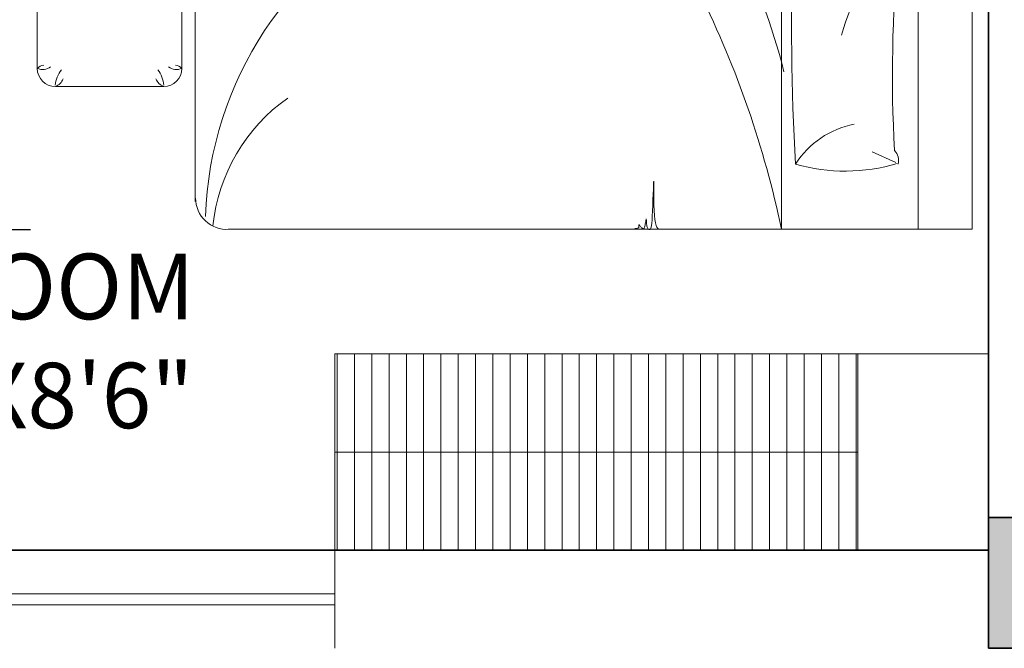
# Model space of a CAD drawing. Units: inches. Extents: x 3321 to 5237, y 11 to 1752.
# Tile 16 of 43: x 4367 to 4458, y 1172 to 1230. Entities that reach past the tile are written whole.
import ezdxf

# ---------------------------------------------------------------- set-up
doc = ezdxf.new("R2010")
doc.units = ezdxf.units.IN
for name, color, linetype, lineweight in [('A-ANNO-DIMS', 2, 'Continuous', 18), ('A-AREA-IDEN', 7, 'Continuous', 18), ('A-COLS', 1, 'Continuous', 35), ('A-FLOR-CASE', 8, 'Continuous', 18), ('A-FLOR-CASE-PATT', 8, 'Continuous', 13), ('A-GLAZ', 5, 'Continuous', 18), ('A-WALL', 7, 'Continuous', 35), ('FUR', 42, 'Continuous', 18)]:
    doc.layers.add(name, color=color, linetype=linetype, lineweight=lineweight)
doc.styles.get("Standard").update_dxf_attribs({"font": 'arial.ttf'})
doc.dimstyles.new('ISO-25', dxfattribs={"dimtxt": 9, "dimasz": 2.5, "dimexe": 1.25, "dimexo": 0.625, "dimtad": 1, "dimdec": 1, "dimlunit": 3, "dimtxsty": 'Standard', "dimcen": 2.5, "dimclrd": 4, "dimclre": 4, "dimclrt": 256, "dimadec": 0, "dimazin": 0, "dimtfac": 1, "dimtdec": 1, "dimtmove": 0, "dimatfit": 3, "dimfxl": 1, "dimarcsym": 0})

# ---------------------------------------------------------------- blocks, each defined once
blk = doc.blocks.new('*X127')
at = {"color": 0}
for p, q in [((3155.9, 8182.9), (3155.9, 8182.9)), ((3147.8, 8143.4), (3147.8, 8143.4)), ((3283, 8049.6), (3283, 8049.6)), ((3209.5, 8023.9), (3209.5, 8023.9)), ((3251.6, 7997), (3251.6, 7997)), ((3154.1, 7950.7), (3154.1, 7950.7))]:
    blk.add_line(p, q, dxfattribs=at)
blk = doc.blocks.new('*X126')
at = {"color": 0}
for p, q in [((3155.9, 8182.9), (3155.9, 8182.9)), ((3139.8, 7939.7), (3139.8, 7939.7))]:
    blk.add_line(p, q, dxfattribs=at)
blk = doc.blocks.new('*X125')
at = {"color": 0}
for p, q in [((3155.9, 8182.9), (3155.9, 8182.9)), ((3139.8, 7939.7), (3139.8, 7939.7))]:
    blk.add_line(p, q, dxfattribs=at)
blk = doc.blocks.new('*X124')
at = {"color": 0}
for p, q in [((3163, 7776.2), (3163, 7776.2)), ((3422.2, 7761.3), (3422.2, 7761.3)), ((3244.3, 7698.6), (3244.3, 7698.6)), ((3340.3, 7689.4), (3340.3, 7689.4)), ((3236.2, 7675.7), (3236.2, 7675.7))]:
    blk.add_line(p, q, dxfattribs=at)
blk = doc.blocks.new('BED1')
for p, q in [((0, -1000), (0, 800)), ((150, 800), (0, 800)), ((150, 800), (150, -1000)), ((2058.7, 800), (150, 800)), ((528, 800), (528, -1000)), ((211.8, 614.9), (277.5, 585.4)), ((2537.2, 404.9), (2237.2, 404.9)), ((2187.2, 354.9), (2187.2, -545.1)), ((2587.2, -545.1), (2587.2, 354.9)), ((2566.3, 178.5), (2565.2, 177.4)), ((2582, 188.1), (2565.4, 174.8)), ((2565.4, 174.8), (2585.7, 165.4)), ((2566.3, -296.8), (2565.2, -297.9)), ((2582, -287.1), (2565.4, -300.5)), ((2565.4, -300.5), (2585.7, -309.9)), ((2237.2, -595.1), (2537.2, -595.1)), ((150, -1000), (0, -1000)), ((150, -1000), (2063.5, -1000))]:
    blk.add_line(p, q)
for points in [[(934, 797.9), (930.9, 797.7), (928.3, 797.4), (926.3, 796.9), (924.9, 796.3), (923.8, 795.6), (923.1, 794.8), (922.7, 793.8), (922.5, 792.7), (922.4, 791.5), (922.5, 790.3), (922.6, 789.2), (922.6, 788.3), (922.6, 787.6), (922.4, 787.3), (922, 787.4), (921.4, 787.9), (920.6, 788.9), (919.5, 790.2), (918.4, 791.6), (917.1, 793.1), (915.9, 794.6), (914.6, 796), (913.3, 797.1), (912.2, 797.9), (911.1, 798.3), (910.1, 798.4), (909.2, 798), (908.3, 797.1), (907.5, 795.8), (906.8, 793.9), (906, 791.4), (905.4, 788.5), (904.8, 785.2), (904.2, 781.7), (903.7, 778.4), (903.2, 775.4), (902.8, 772.9), (902.5, 771.3), (902.3, 770.6), (902.1, 771.2), (902, 772.8), (901.8, 775.2), (901.7, 778.1), (901.5, 781.5), (901.2, 785), (900.8, 788.4), (900.2, 791.5), (899.5, 794.1), (898.6, 796.2), (897.6, 797.9), (896.5, 799.2), (895.3, 800), (894.1, 800.5), (893, 800.7), (891.9, 800.5), (890.9, 800.1), (890, 799), (889.1, 797.1), (888.3, 794), (887.6, 789.3), (886.9, 782.9), (886.2, 774.2), (885.5, 763.1), (884.8, 749.5), (884.2, 734.2), (883.6, 718.3), (883, 702.8), (882.5, 688.8), (882, 677.5), (881.7, 669.8), (881.5, 666.9), (881.3, 669.4), (881.3, 676.7), (881.3, 687.8), (881.2, 701.5), (881.1, 716.8), (880.8, 732.6), (880.2, 748), (879.4, 761.8), (878.3, 773.2), (876.9, 782.2), (875.1, 789.2), (872.9, 794.4), (870.3, 798), (869, 799)], [(2150, -913.5), (2150, 723.2)], [(2327.6, 182.3), (2530, 185.9), (2550.8, 181.9), (2561.7, 179), (2566, 176.7), (2566.9, 174.4), (2566.3, 171.9), (2562, 169.2), (2550.3, 166.5), (2527.7, 163.9), (2490.6, 161.8), (2345.5, 160.2), (2317.8, 158.5)], [(494.7, 3.1), (458.9, 95.3)], [(2149.7, -259.9), (2150, -268.4), (2150.1, -274.1), (2150.1, -278.1), (2150, -281.4), (2149.8, -284), (2149.5, -286.1), (2149.1, -287.8), (2148.7, -289), (2148.1, -289.9), (2147.4, -290.5), (2146.6, -290.8), (2145.6, -291), (2144.6, -291), (2143.6, -291), (2142.7, -290.9), (2141.9, -290.9), (2141.4, -290.9), (2141.1, -291), (2141.2, -291.4), (2141.7, -291.9), (2142.5, -292.6), (2143.5, -293.4), (2144.7, -294.4), (2146, -295.4), (2147.2, -296.5), (2148.4, -297.6), (2149.3, -298.6), (2150, -299.6), (2150.3, -300.5), (2150.4, -301.3), (2150, -302.1), (2149.3, -302.8), (2148.2, -303.5), (2146.6, -304.1), (2144.6, -304.7), (2142.1, -305.2), (2139.3, -305.7), (2136.5, -306.2), (2133.7, -306.6), (2131.2, -307), (2129.2, -307.3), (2127.8, -307.6), (2127.3, -307.8), (2127.7, -308), (2129, -308.1), (2131, -308.2), (2133.5, -308.3), (2136.3, -308.5), (2139.2, -308.7), (2142, -309), (2144.6, -309.5), (2146.8, -310.1), (2148.6, -310.9), (2150, -311.7), (2151, -312.7), (2151.7, -313.6), (2152.1, -314.6), (2152.3, -315.6), (2152.2, -316.5), (2151.8, -317.3), (2150.9, -318.1), (2149.3, -318.8), (2146.7, -319.4), (2142.8, -320), (2137.4, -320.6), (2130.2, -321.2), (2121, -321.8), (2109.7, -322.3), (2096.9, -322.9), (2083.6, -323.4), (2070.7, -323.9), (2059.1, -324.3), (2049.6, -324.7), (2043.2, -325), (2040.8, -325.2), (2042.9, -325.3), (2049, -325.3), (2058.2, -325.3), (2069.6, -325.4), (2082.3, -325.5), (2095.6, -325.8), (2108.4, -326.2), (2119.9, -326.8), (2129.4, -327.8), (2136.9, -329), (2142.7, -330.5), (2147, -332.3), (2150, -334.4), (2150.9, -335.6)], [(2246.5, -294.4), (2530, -289.4), (2550.8, -293.4), (2561.7, -296.3), (2566, -298.6), (2566.9, -300.8), (2566.3, -303.4), (2562, -306.1), (2550.3, -308.8), (2527.7, -311.3), (2490.6, -313.5), (2345.5, -315), (2238.6, -321.8)], [(1733.7, -998.3), (1731.1, -998.1), (1729, -997.8), (1727.4, -997.4), (1726.1, -997), (1725.2, -996.4), (1724.7, -995.7), (1724.3, -994.8), (1724.1, -993.9), (1724.1, -992.9), (1724.1, -991.9), (1724.2, -991), (1724.2, -990.2), (1724.2, -989.7), (1724.1, -989.4), (1723.8, -989.5), (1723.2, -990), (1722.5, -990.8), (1721.7, -991.8), (1720.7, -993), (1719.7, -994.3), (1718.6, -995.5), (1717.5, -996.6), (1716.5, -997.6), (1715.5, -998.3), (1714.6, -998.6), (1713.8, -998.6), (1713, -998.3), (1712.3, -997.6), (1711.7, -996.5), (1711, -994.9), (1710.4, -992.9), (1709.9, -990.4), (1709.4, -987.6), (1708.9, -984.8), (1708.5, -982), (1708.1, -979.5), (1707.8, -977.4), (1707.5, -976.1), (1707.3, -975.5), (1707.1, -976), (1707, -977.3), (1706.9, -979.3), (1706.8, -981.8), (1706.7, -984.6), (1706.4, -987.5), (1706.1, -990.3), (1705.6, -992.9), (1705, -995.1), (1704.2, -996.9), (1703.4, -998.3), (1702.4, -999.3), (1701.5, -1000), (1700.5, -1000.4), (1699.6, -1000.6), (1698.7, -1000.4), (1697.8, -1000.1), (1697, -999.2), (1696.3, -997.6), (1695.7, -995), (1695.1, -991.1), (1694.5, -985.7), (1693.9, -978.5), (1693.3, -969.3), (1692.8, -957.9), (1692.2, -945.2), (1691.7, -931.9), (1691.2, -919), (1690.8, -907.4), (1690.4, -897.9), (1690.1, -891.5), (1689.9, -889.1), (1689.8, -891.2), (1689.8, -897.3), (1689.8, -906.5), (1689.7, -917.9), (1689.6, -930.6), (1689.4, -943.8), (1688.9, -956.6), (1688.3, -968.1), (1687.3, -977.6), (1686.1, -985.2), (1684.6, -991), (1682.8, -995.3), (1680.7, -998.3), (1679.6, -999.2)]]:
    blk.add_lwpolyline(points)
for points in [[(489.2, 619.6, 0.144019), (207.6, 617.9, 0.248643)], [(205.5, 619.6, 0.267769), (215.1, 582.4, -0.037739), (204.3, 21.8, 0.684696), (236.7, 5.5, -0.060702), (497.2, 0.1, -0.046649), (225.9, 3.1, -1.318436)], [(497.2, 0.1, 0.021276), (489.2, 619.6, -0.206383), (326.6, 509.4, 0.237198)], [(211.8, 12.8, 0.143972), (361.6, 262.9, 1.292232)], [(886.4, -150, -0.069098), (985, -66.5, 0.658965), (982.1, -48.7, -0.049789), (927.4, -29, -0.103757), (896.6, -5.4, 0.055725), (800.9, 83.3, -0.11866), (782.7, 104.9, 0.016811), (761.6, 143.9, 0.70791), (748.3, 144, -0.16964), (551.9, -96.6, 0.664036), (554, -110.7, 0.023706), (627, -144.7, -0.134834), (683.2, -188, 0.012748), (746.3, -267.4)], [(969.1, -259.1, 0.263265), (936.3, -236.9, -0.026108), (909.2, -233.2, 0.027613), (945.1, -234.2, -0.089259), (872.7, -120, 0.662242), (857.6, -119.3, -0.162037), (651.8, -332.7, 0.676499), (654, -354.5, -0.160513), (722.9, -401.5, 0.07473), (773.5, -450.3, -0.187721), (845.5, -559.9, 0.70791), (858.8, -561.4, -0.010003), (898.6, -497.3, -0.113819), (947.3, -450.2, 0.099539), (1032.5, -372.4, -0.173425), (1070.9, -346.4, 0.589988), (1076.2, -326.1, 0.137312), (923.9, -245.9, 0.137312)], [(489.2, -168.2, 0.144019), (207.6, -169.9, 0.248643)], [(205.5, -168.2, 0.267769), (215.1, -205.4, -0.037739), (204.3, -766, 0.684696), (236.7, -782.3, -0.060702), (497.2, -787.7, -0.046649), (225.9, -784.7, -1.318436)], [(497.2, -787.7, 0.021276), (489.2, -168.2, -0.206383), (326.6, -278.4, 0.237198)], [(1446, -733.4, -0.095039), (652.8, -1001.7)]]:
    blk.add_lwpolyline(points, format="xyb")
for centre, radius, start, end in [((3208.8, 1363.3), 2739.4, 191.8679, 206.3247), ((1608.1, 842.5), 496.3, 305.1901, 354.0206), ((2062.7, 713.7), 86.5, 0, 93.5376), ((1138.6, 793.9), 983.2, 294.6078, 358.3033), ((2237.2, 354.9), 50, 90, 180), ((2321.1, 409.7), 84.5, 185.6196, 217.1396), ((2227.5, 373.5), 32.8, 17.833, 72.8005), ((2546.9, 373.5), 32.8, 107.1995, 162.167), ((2453.3, 409.7), 84.5, 322.8604, 354.3804), ((2537.2, 354.9), 50, 0, 90), ((2098.7, 754.7), 1625, 193.905, 207.8169), ((2201.9, 323.3), 34.8, 50.8413, 114.9586), ((2212.2, 381.5), 36.5, 226.8095, 258.3841), ((2572.5, 323.3), 34.8, 65.0414, 129.1587), ((2562.2, 381.5), 36.5, 281.6159, 313.1905), ((751.8, 88.7), 34.9, 336.8352, 27.7218), ((684.2, 86), 100.3, 353.675, 10.882), ((1074.1, 198.8), 306.1, 197.8602, 241.5122), ((341.4, -277.7), 318.5, 60.7125, 115.009), ((978.5, -68.6), 14.3, 39.7097, 85.9506), ((983.7, -79.5), 20.8, 73.7967, 130.4566), ((602.5, -324), 198.6, 43.2035, 95.0556), ((3208.8, 1363.3), 2739.4, 212.9314, 216.951), ((981.1, -281.8), 131.1, 164.0372, 243.4536), ((980, -379), 163.4, 152.6104, 209.361), ((3208.8, 1363.3), 2739.4, 218.6329, 229.9449), ((2098.7, 754.7), 1625, 226.5887, 246.3156), ((3402.5, -342.9), 1408.5, 182.9917, 205.6819), ((-34.4, -471.2), 376.5, 312.0118, 350.9635), ((2178, -513.5), 33, 286.1827, 338.1386), ((2188.1, -476.2), 73, 269.4513, 322.8027), ((2572.5, -513.6), 34.8, 230.8413, 294.9586), ((2562.2, -571.8), 36.5, 46.8095, 78.3841), ((2237.2, -545.1), 50, 180, 270), ((2271.1, -580.9), 35.8, 148.9055, 197.5541), ((2453.3, -600), 84.5, 5.6196, 37.1396), ((2537.2, -545.1), 50, 270, 0), ((2546.9, -563.8), 32.8, 197.833, 252.8005), ((375.7, -807.4), 128.2, 17.4073, 88.5129), ((341.4, -1065.5), 318.5, 60.7125, 115.009), ((1929.1, -1126), 250.5, 37.8553, 88.4405), ((2063.5, -913.5), 86.5, 270, 0)]:
    blk.add_arc(centre, radius, start, end)
for name in ['*X126', '*X125', '*X127', '*X124']:
    blk.add_blockref(name, (-2425.3, -8101.4))
blk = doc.blocks.new('COL-9X12-FURN-PLAN')
h = blk.add_hatch(color=256)
h.dxf.hatch_style = 1
h.paths.add_polyline_path([(0, 12), (0, 0), (9, 0), (9, 12)])
blk.add_lwpolyline([(0, 0), (9, 0), (9, 12), (0, 12)], close=True)
blk = doc.blocks.new('WIN-48IN-9IN-WALL')
for p, q in [((0, 0), (0, 9)), ((48, 0), (48, 9)), ((0, 5), (48, 5)), ((0, 4), (48, 4))]:
    blk.add_line(p, q)
blk = doc.blocks.new('*D196')
at = {"layer": 'A-ANNO-DIMS', "color": 4, "lineweight": -2, "transparency": 16777216}
for p, q in [((4368.448, 1270.54), (4354.95, 1270.54)), ((4356.2, 1268.04), (4356.2, 1213.226)), ((4368.448, 1210.726), (4354.95, 1210.726))]:
    blk.add_line(p, q, dxfattribs=at)
at = {"layer": 'A-ANNO-DIMS', "color": 4, "transparency": 16777216}
for points in [[(4355.783, 1268.04), (4356.616, 1268.04), (4356.2, 1270.54)], [(4355.783, 1213.226), (4356.616, 1213.226), (4356.2, 1210.726)]]:
    blk.add_solid(points, dxfattribs=at)
at = {"layer": 'Defpoints', "color": 0, "transparency": 16777216}
for p in [(4369.073, 1270.54), (4356.2, 1210.726), (4369.073, 1210.726)]:
    blk.add_point(p, dxfattribs=at)
at = {"layer": 'A-ANNO-DIMS', "transparency": 16777216, "insert": (4350.98, 1240.633), "char_height": 9, "attachment_point": 5, "rotation": 90}
blk.add_mtext('5\'-0"', dxfattribs=at)

msp = doc.modelspace()

# ---------------------------------------------------------------- hatches: boundary and pattern name
at = {"layer": 'A-FLOR-CASE-PATT'}
h = msp.add_hatch(dxfattribs=at)
h.set_pattern_fill('ANSI31', color=256, scale=0.5, angle=45)
h.set_pattern_definition([(90, (-735.7874, -1e-13), (-1.5875, 0), [])])
h.paths.add_polyline_path([(4396.386, 1199.339), (4396.386, 1181.339), (4444.386, 1181.339), (4444.386, 1199.339)])

# ---------------------------------------------------------------- linework, layer by layer
at = {"layer": 'A-FLOR-CASE'}
for p, q in [((4396.386, 1199.339), (4456.386, 1199.339)), ((4396.386, 1181.339), (4396.386, 1199.339)), ((4444.386, 1199.339), (4444.386, 1181.339)), ((4444.386, 1190.339), (4396.386, 1190.339))]:
    msp.add_line(p, q, dxfattribs=at)
at = {"layer": 'A-WALL'}
for p in [(4456.386, 1283.339), (4336.386, 1181.339)]:
    msp.add_line(p, (4456.386, 1181.339), dxfattribs=at)

# ---------------------------------------------------------------- block references
at = {"layer": 'A-COLS'}
msp.add_blockref('COL-9X12-FURN-PLAN', (4456.386, 1172.339), dxfattribs=at)
at = {"layer": 'A-GLAZ'}
msp.add_blockref('WIN-48IN-9IN-WALL', (4348.386, 1172.339), dxfattribs=at)
at = {"layer": 'FUR', "xscale": 0.0331718847221821, "yscale": 0.0331718847221821, "zscale": 0.0331718847221821, "rotation": 180}
msp.add_blockref('BED1', (4454.896, 1237.313), dxfattribs=at)

# ---------------------------------------------------------------- texts
at = {"layer": 'A-AREA-IDEN', "insert": (4343.699, 1208.532), "char_height": 6, "attachment_point": 1}
msp.add_mtext_dynamic_manual_height_columns('BEDROOM\\P10\'0"X8\'6"', width=97.3114, gutter_width=25, heights=[0], dxfattribs=at)

# ---------------------------------------------------------------- dimensions: what is measured, and where the dimension line sits
at = {"layer": 'A-ANNO-DIMS'}
dim = msp.add_linear_dim(base=(4356.2, 1210.726), p1=(4369.073, 1270.54), p2=(4369.073, 1210.726), angle=270, dimstyle='ISO-25', override={"dimdec": 1, "dimlfac": 1, "dimrnd": 0, "dimzin": 1, "dimdsep": 46, "dimlunit": 4, "dimfrac": 2}, dxfattribs=at)
dim.commit()
dim.dimension.update_dxf_attribs({"geometry": '*D196', "text_midpoint": (4350.98, 1240.633)})

doc.saveas('drawing.dxf')
